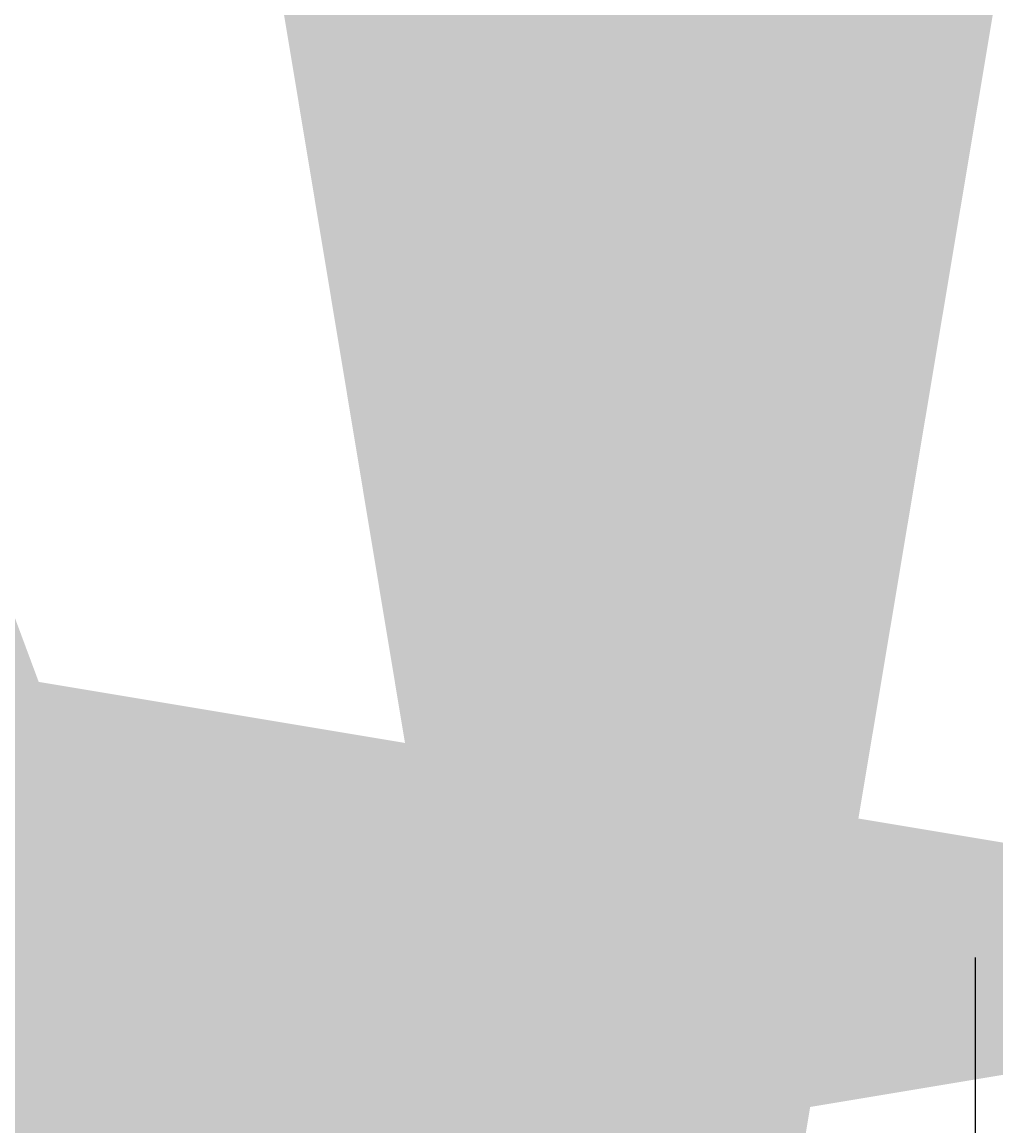
# Model space of a CAD drawing. Units: millimetres. Extents: x -22994 to 29398, y -19990 to 20176.
# Tile 26 of 135: x -44 to 99, y 180 to 341. Entities that reach past the tile are written whole.
import ezdxf

# ---------------------------------------------------------------- set-up
doc = ezdxf.new("R2010")
doc.units = ezdxf.units.MM
doc.header["$MEASUREMENT"] = 0
doc.layers.add('M-DIMS', color=2, linetype='Continuous', lineweight=18)
doc.styles.get("Standard").update_dxf_attribs({"font": 'arial.ttf'})
doc.dimstyles.get("Standard").update_dxf_attribs({"dimtxt": 0.18, "dimasz": 10000, "dimexe": 0.18, "dimexo": 0.0625, "dimgap": 0.09, "dimtad": 0, "dimtih": 1, "dimtoh": 1, "dimdec": 0, "dimzin": 0, "dimdsep": 46, "dimtxsty": 'Standard', "dimcen": 0.09, "dimadec": 0, "dimazin": 0, "dimtfac": 1, "dimtdec": 0, "dimtofl": 0, "dimtmove": 0, "dimatfit": 3, "dimfxl": 1, "dimtolj": 1, "dimtzin": 0, "dimlwd": 30, "dimarcsym": 0})

# ---------------------------------------------------------------- blocks, each defined once
blk = doc.blocks.new('*D2')
at = {"layer": 'Defpoints', "color": 0, "transparency": 16777216}
for p in [(6.68, 10.27), (290.85, 10.27), (290.85, -5.08)]:
    blk.add_point(p, dxfattribs=at)
at = {"layer": 'M-DIMS', "color": 0, "lineweight": -2, "transparency": 16777216}
for p, q in [((6.68, 10.21), (6.68, -5.26)), ((290.85, 10.21), (290.85, -5.26))]:
    blk.add_line(p, q, dxfattribs=at)
at = {"layer": 'M-DIMS', "color": 0, "lineweight": 30, "transparency": 16777216}
for p, q in [((-9993.32, -5.08), (-19993.32, -5.08)), ((10290.85, -5.08), (20290.85, -5.08))]:
    blk.add_line(p, q, dxfattribs=at)
at = {"layer": 'M-DIMS', "color": 0, "transparency": 16777216}
for points in [[(-9993.32, 1661.59), (-9993.32, -1671.75), (6.68, -5.08)], [(10290.85, 1661.59), (10290.85, -1671.75), (290.85, -5.08)]]:
    blk.add_solid(points, dxfattribs=at)
at = {"layer": 'M-DIMS', "color": 0, "transparency": 16777216, "insert": (148.76, -5.08), "char_height": 0.18, "attachment_point": 5}
blk.add_mtext('\\A1;284.2', dxfattribs=at)
blk = doc.blocks.new('*D3')
at = {"layer": 'Defpoints', "color": 0, "transparency": 16777216}
for p in [(110.26, 204.17), (110.26, 176.37), (95.83, 127.97)]:
    blk.add_point(p, dxfattribs=at)
at = {"layer": 'M-DIMS', "color": 0, "lineweight": 30, "transparency": 16777216}
for p, q in [((-9904.17, 204.17), (-19904.17, 204.17)), ((10110.26, 204.17), (20110.26, 204.17))]:
    blk.add_line(p, q, dxfattribs=at)
at = {"layer": 'M-DIMS', "color": 0, "lineweight": -2, "transparency": 16777216}
for p, q in [((95.83, 128.03), (95.83, 204.35)), ((110.26, 176.43), (110.26, 204.35))]:
    blk.add_line(p, q, dxfattribs=at)
at = {"layer": 'M-DIMS', "color": 0, "transparency": 16777216}
for points in [[(-9904.17, 1870.83), (-9904.17, -1462.5), (95.83, 204.17)], [(10110.26, 1870.83), (10110.26, -1462.5), (110.26, 204.17)]]:
    blk.add_solid(points, dxfattribs=at)
at = {"layer": 'M-DIMS', "color": 0, "transparency": 16777216, "insert": (103.05, 204.17), "char_height": 0.18, "attachment_point": 5}
blk.add_mtext('\\A1;14.432', dxfattribs=at)
blk = doc.blocks.new('*D4')
at = {"layer": 'Defpoints', "color": 0, "transparency": 16777216}
for p in [(116.26, 204.17), (110.26, 176.37), (116.26, 176.37)]:
    blk.add_point(p, dxfattribs=at)
at = {"layer": 'M-DIMS', "color": 0, "lineweight": 30, "transparency": 16777216}
for p, q in [((-9889.74, 204.17), (-19889.74, 204.17)), ((10116.26, 204.17), (20116.26, 204.17))]:
    blk.add_line(p, q, dxfattribs=at)
at = {"layer": 'M-DIMS', "color": 0, "lineweight": -2, "transparency": 16777216}
for p, q in [((110.26, 176.43), (110.26, 204.35)), ((116.26, 176.43), (116.26, 204.35))]:
    blk.add_line(p, q, dxfattribs=at)
at = {"layer": 'M-DIMS', "color": 0, "transparency": 16777216}
for points in [[(-9889.74, 1870.83), (-9889.74, -1462.5), (110.26, 204.17)], [(10116.26, 1870.83), (10116.26, -1462.5), (116.26, 204.17)]]:
    blk.add_solid(points, dxfattribs=at)
at = {"layer": 'M-DIMS', "color": 0, "transparency": 16777216, "insert": (113.26, 204.17), "char_height": 0.18, "attachment_point": 5}
blk.add_mtext('\\A1;6', dxfattribs=at)
blk = doc.blocks.new('*D5')
at = {"layer": 'Defpoints', "color": 0, "transparency": 16777216}
for p in [(181.26, 204.17), (116.26, 176.37), (181.26, 176.37)]:
    blk.add_point(p, dxfattribs=at)
at = {"layer": 'M-DIMS', "color": 0, "lineweight": 30, "transparency": 16777216}
for p, q in [((-9883.74, 204.17), (-19883.74, 204.17)), ((10181.26, 204.17), (20181.26, 204.17))]:
    blk.add_line(p, q, dxfattribs=at)
at = {"layer": 'M-DIMS', "color": 0, "lineweight": -2, "transparency": 16777216}
for p, q in [((116.26, 176.43), (116.26, 204.35)), ((181.26, 176.43), (181.26, 204.35))]:
    blk.add_line(p, q, dxfattribs=at)
at = {"layer": 'M-DIMS', "color": 0, "transparency": 16777216}
for points in [[(-9883.74, 1870.83), (-9883.74, -1462.5), (116.26, 204.17)], [(10181.26, 1870.83), (10181.26, -1462.5), (181.26, 204.17)]]:
    blk.add_solid(points, dxfattribs=at)
at = {"layer": 'M-DIMS', "color": 0, "transparency": 16777216, "insert": (148.76, 204.17), "char_height": 0.18, "attachment_point": 5}
blk.add_mtext('\\A1;65', dxfattribs=at)
blk = doc.blocks.new('*D6')
at = {"layer": 'Defpoints', "color": 0, "transparency": 16777216}
for p in [(187.26, 204.17), (181.26, 176.37), (187.26, 176.37)]:
    blk.add_point(p, dxfattribs=at)
at = {"layer": 'M-DIMS', "color": 0, "lineweight": 30, "transparency": 16777216}
for p, q in [((-9818.74, 204.17), (-19818.74, 204.17)), ((10187.26, 204.17), (20187.26, 204.17))]:
    blk.add_line(p, q, dxfattribs=at)
at = {"layer": 'M-DIMS', "color": 0, "lineweight": -2, "transparency": 16777216}
for p, q in [((181.26, 176.43), (181.26, 204.35)), ((187.26, 176.43), (187.26, 204.35))]:
    blk.add_line(p, q, dxfattribs=at)
at = {"layer": 'M-DIMS', "color": 0, "transparency": 16777216}
for points in [[(-9818.74, 1870.83), (-9818.74, -1462.5), (181.26, 204.17)], [(10187.26, 1870.83), (10187.26, -1462.5), (187.26, 204.17)]]:
    blk.add_solid(points, dxfattribs=at)
at = {"layer": 'M-DIMS', "color": 0, "transparency": 16777216, "insert": (184.26, 204.17), "char_height": 0.18, "attachment_point": 5}
blk.add_mtext('\\A1;6', dxfattribs=at)
blk = doc.blocks.new('*D7')
at = {"layer": 'Defpoints', "color": 0, "transparency": 16777216}
for p in [(201.7, 204.17), (187.26, 176.37), (201.7, 127.97)]:
    blk.add_point(p, dxfattribs=at)
at = {"layer": 'M-DIMS', "color": 0, "lineweight": 30, "transparency": 16777216}
for p, q in [((-9812.74, 204.17), (-19812.74, 204.17)), ((10201.7, 204.17), (20201.7, 204.17))]:
    blk.add_line(p, q, dxfattribs=at)
at = {"layer": 'M-DIMS', "color": 0, "lineweight": -2, "transparency": 16777216}
for p, q in [((187.26, 176.43), (187.26, 204.35)), ((201.7, 128.03), (201.7, 204.35))]:
    blk.add_line(p, q, dxfattribs=at)
at = {"layer": 'M-DIMS', "color": 0, "transparency": 16777216}
for points in [[(-9812.74, 1870.83), (-9812.74, -1462.5), (187.26, 204.17)], [(10201.7, 1870.83), (10201.7, -1462.5), (201.7, 204.17)]]:
    blk.add_solid(points, dxfattribs=at)
at = {"layer": 'M-DIMS', "color": 0, "transparency": 16777216, "insert": (194.48, 204.17), "char_height": 0.18, "attachment_point": 5}
blk.add_mtext('\\A1;14.432', dxfattribs=at)
blk = doc.blocks.new('*D8')
at = {"layer": 'Defpoints', "color": 0, "transparency": 16777216}
for p in [(227.65, 204.17), (227.65, 146.73), (201.7, 127.97)]:
    blk.add_point(p, dxfattribs=at)
at = {"layer": 'M-DIMS', "color": 0, "lineweight": 30, "transparency": 16777216}
for p, q in [((-9798.3, 204.17), (-19798.3, 204.17)), ((10227.65, 204.17), (20227.65, 204.17))]:
    blk.add_line(p, q, dxfattribs=at)
at = {"layer": 'M-DIMS', "color": 0, "lineweight": -2, "transparency": 16777216}
for p, q in [((201.7, 128.03), (201.7, 204.35)), ((227.65, 146.79), (227.65, 204.35))]:
    blk.add_line(p, q, dxfattribs=at)
at = {"layer": 'M-DIMS', "color": 0, "transparency": 16777216}
for points in [[(-9798.3, 1870.83), (-9798.3, -1462.5), (201.7, 204.17)], [(10227.65, 1870.83), (10227.65, -1462.5), (227.65, 204.17)]]:
    blk.add_solid(points, dxfattribs=at)
at = {"layer": 'M-DIMS', "color": 0, "transparency": 16777216, "insert": (214.67, 204.17), "char_height": 0.18, "attachment_point": 5}
blk.add_mtext('\\A1;25.95', dxfattribs=at)
blk = doc.blocks.new('*D9')
at = {"layer": 'Defpoints', "color": 0, "transparency": 16777216}
for p in [(187.26, 176.37), (306.2, 176.37), (290.85, 10.27)]:
    blk.add_point(p, dxfattribs=at)
at = {"layer": 'M-DIMS', "color": 0, "lineweight": 30, "transparency": 16777216}
for p, q in [((306.2, 10176.37), (306.2, 20176.37)), ((306.2, -9989.73), (306.2, -19989.73))]:
    blk.add_line(p, q, dxfattribs=at)
at = {"layer": 'M-DIMS', "color": 0, "lineweight": -2, "transparency": 16777216}
for p, q in [((187.33, 176.37), (306.38, 176.37)), ((290.91, 10.27), (306.38, 10.27))]:
    blk.add_line(p, q, dxfattribs=at)
at = {"layer": 'M-DIMS', "color": 0, "transparency": 16777216}
for points in [[(-1360.46, 10176.37), (1972.87, 10176.37), (306.2, 176.37)], [(-1360.46, -9989.73), (1972.87, -9989.73), (306.2, 10.27)]]:
    blk.add_solid(points, dxfattribs=at)
at = {"layer": 'M-DIMS', "color": 0, "transparency": 16777216, "insert": (306.2, 93.32), "char_height": 0.18, "attachment_point": 5}
blk.add_mtext('\\A1;166.1', dxfattribs=at)
blk = doc.blocks.new('*D10')
at = {"layer": 'Defpoints', "color": 0, "transparency": 16777216}
for p in [(125.65, 136.07), (133.35, 136.07), (133.35, -5.08)]:
    blk.add_point(p, dxfattribs=at)
at = {"layer": 'M-DIMS', "color": 0, "lineweight": -2, "transparency": 16777216}
for p, q in [((125.65, 136.01), (125.65, -5.26)), ((133.35, 136.01), (133.35, -5.26))]:
    blk.add_line(p, q, dxfattribs=at)
at = {"layer": 'M-DIMS', "color": 0, "lineweight": 30, "transparency": 16777216}
for p, q in [((-9874.35, -5.08), (-19874.35, -5.08)), ((10133.35, -5.08), (20133.35, -5.08))]:
    blk.add_line(p, q, dxfattribs=at)
at = {"layer": 'M-DIMS', "color": 0, "transparency": 16777216}
for points in [[(-9874.35, 1661.59), (-9874.35, -1671.75), (125.65, -5.08)], [(10133.35, 1661.59), (10133.35, -1671.75), (133.35, -5.08)]]:
    blk.add_solid(points, dxfattribs=at)
at = {"layer": 'M-DIMS', "color": 0, "transparency": 16777216, "insert": (129.5, -5.08), "char_height": 0.18, "attachment_point": 5}
blk.add_mtext('\\A1;7.696', dxfattribs=at)
blk = doc.blocks.new('*D11')
at = {"layer": 'Defpoints', "color": 0, "transparency": 16777216}
for p in [(133.35, 136.07), (135.65, 136.07), (135.65, -5.08)]:
    blk.add_point(p, dxfattribs=at)
at = {"layer": 'M-DIMS', "color": 0, "lineweight": -2, "transparency": 16777216}
for p, q in [((133.35, 136.01), (133.35, -5.26)), ((135.65, 136.01), (135.65, -5.26))]:
    blk.add_line(p, q, dxfattribs=at)
at = {"layer": 'M-DIMS', "color": 0, "lineweight": 30, "transparency": 16777216}
for p, q in [((-9866.65, -5.08), (-19866.65, -5.08)), ((10135.65, -5.08), (20135.65, -5.08))]:
    blk.add_line(p, q, dxfattribs=at)
at = {"layer": 'M-DIMS', "color": 0, "transparency": 16777216}
for points in [[(-9866.65, 1661.59), (-9866.65, -1671.75), (133.35, -5.08)], [(10135.65, 1661.59), (10135.65, -1671.75), (135.65, -5.08)]]:
    blk.add_solid(points, dxfattribs=at)
at = {"layer": 'M-DIMS', "color": 0, "transparency": 16777216, "insert": (134.5, -5.08), "char_height": 0.18, "attachment_point": 5}
blk.add_mtext('\\A1;2.304', dxfattribs=at)
blk = doc.blocks.new('*D12')
at = {"layer": 'Defpoints', "color": 0, "transparency": 16777216}
for p in [(135.65, 136.07), (145.65, 136.07), (145.65, -5.08)]:
    blk.add_point(p, dxfattribs=at)
at = {"layer": 'M-DIMS', "color": 0, "lineweight": -2, "transparency": 16777216}
for p, q in [((135.65, 136.01), (135.65, -5.26)), ((145.65, 136.01), (145.65, -5.26))]:
    blk.add_line(p, q, dxfattribs=at)
at = {"layer": 'M-DIMS', "color": 0, "lineweight": 30, "transparency": 16777216}
for p, q in [((-9864.35, -5.08), (-19864.35, -5.08)), ((10145.65, -5.08), (20145.65, -5.08))]:
    blk.add_line(p, q, dxfattribs=at)
at = {"layer": 'M-DIMS', "color": 0, "transparency": 16777216}
for points in [[(-9864.35, 1661.59), (-9864.35, -1671.75), (135.65, -5.08)], [(10145.65, 1661.59), (10145.65, -1671.75), (145.65, -5.08)]]:
    blk.add_solid(points, dxfattribs=at)
at = {"layer": 'M-DIMS', "color": 0, "transparency": 16777216, "insert": (140.65, -5.08), "char_height": 0.18, "attachment_point": 5}
blk.add_mtext('\\A1;10', dxfattribs=at)
blk = doc.blocks.new('*D13')
at = {"layer": 'Defpoints', "color": 0, "transparency": 16777216}
for p in [(145.65, 136.07), (155.65, 136.07), (155.65, -5.08)]:
    blk.add_point(p, dxfattribs=at)
at = {"layer": 'M-DIMS', "color": 0, "lineweight": -2, "transparency": 16777216}
for p, q in [((145.65, 136.01), (145.65, -5.26)), ((155.65, 136.01), (155.65, -5.26))]:
    blk.add_line(p, q, dxfattribs=at)
at = {"layer": 'M-DIMS', "color": 0, "lineweight": 30, "transparency": 16777216}
for p, q in [((-9854.35, -5.08), (-19854.35, -5.08)), ((10155.65, -5.08), (20155.65, -5.08))]:
    blk.add_line(p, q, dxfattribs=at)
at = {"layer": 'M-DIMS', "color": 0, "transparency": 16777216}
for points in [[(-9854.35, 1661.59), (-9854.35, -1671.75), (145.65, -5.08)], [(10155.65, 1661.59), (10155.65, -1671.75), (155.65, -5.08)]]:
    blk.add_solid(points, dxfattribs=at)
at = {"layer": 'M-DIMS', "color": 0, "transparency": 16777216, "insert": (150.65, -5.08), "char_height": 0.18, "attachment_point": 5}
blk.add_mtext('\\A1;10', dxfattribs=at)
blk = doc.blocks.new('*D14')
at = {"layer": 'Defpoints', "color": 0, "transparency": 16777216}
for p in [(155.65, 136.07), (165.65, 136.07), (165.65, -5.08)]:
    blk.add_point(p, dxfattribs=at)
at = {"layer": 'M-DIMS', "color": 0, "lineweight": -2, "transparency": 16777216}
for p, q in [((155.65, 136.01), (155.65, -5.26)), ((165.65, 136.01), (165.65, -5.26))]:
    blk.add_line(p, q, dxfattribs=at)
at = {"layer": 'M-DIMS', "color": 0, "lineweight": 30, "transparency": 16777216}
for p, q in [((-9844.35, -5.08), (-19844.35, -5.08)), ((10165.65, -5.08), (20165.65, -5.08))]:
    blk.add_line(p, q, dxfattribs=at)
at = {"layer": 'M-DIMS', "color": 0, "transparency": 16777216}
for points in [[(-9844.35, 1661.59), (-9844.35, -1671.75), (155.65, -5.08)], [(10165.65, 1661.59), (10165.65, -1671.75), (165.65, -5.08)]]:
    blk.add_solid(points, dxfattribs=at)
at = {"layer": 'M-DIMS', "color": 0, "transparency": 16777216, "insert": (160.65, -5.08), "char_height": 0.18, "attachment_point": 5}
blk.add_mtext('\\A1;10', dxfattribs=at)
blk = doc.blocks.new('*D15')
at = {"layer": 'Defpoints', "color": 0, "transparency": 16777216}
for p in [(173.35, 154.79), (173.35, 136.07), (306.2, 136.07)]:
    blk.add_point(p, dxfattribs=at)
at = {"layer": 'M-DIMS', "color": 0, "lineweight": 30, "transparency": 16777216}
for p, q in [((306.2, 10154.79), (306.2, 20154.79)), ((306.2, -9863.93), (306.2, -19863.93))]:
    blk.add_line(p, q, dxfattribs=at)
at = {"layer": 'M-DIMS', "color": 0, "lineweight": -2, "transparency": 16777216}
for p, q in [((173.41, 154.79), (306.38, 154.79)), ((173.41, 136.07), (306.38, 136.07))]:
    blk.add_line(p, q, dxfattribs=at)
at = {"layer": 'M-DIMS', "color": 0, "transparency": 16777216}
for points in [[(-1360.46, 10154.79), (1972.87, 10154.79), (306.2, 154.79)], [(-1360.46, -9863.93), (1972.87, -9863.93), (306.2, 136.07)]]:
    blk.add_solid(points, dxfattribs=at)
at = {"layer": 'M-DIMS', "color": 0, "transparency": 16777216, "insert": (306.2, 145.43), "char_height": 0.18, "attachment_point": 5}
blk.add_mtext('\\A1;18.717', dxfattribs=at)
blk = doc.blocks.new('*D16')
at = {"layer": 'Defpoints', "color": 0, "transparency": 16777216}
for p in [(120.17, 204.17), (110.47, 48.03), (120.17, 48.03)]:
    blk.add_point(p, dxfattribs=at)
at = {"layer": 'M-DIMS', "color": 0, "lineweight": 30, "transparency": 16777216}
for p, q in [((-9889.53, 204.17), (-19889.53, 204.17)), ((10120.17, 204.17), (20120.17, 204.17))]:
    blk.add_line(p, q, dxfattribs=at)
at = {"layer": 'M-DIMS', "color": 0, "lineweight": -2, "transparency": 16777216}
for p, q in [((110.47, 48.1), (110.47, 204.35)), ((120.17, 48.1), (120.17, 204.35))]:
    blk.add_line(p, q, dxfattribs=at)
at = {"layer": 'M-DIMS', "color": 0, "transparency": 16777216}
for points in [[(-9889.53, 1870.83), (-9889.53, -1462.5), (110.47, 204.17)], [(10120.17, 1870.83), (10120.17, -1462.5), (120.17, 204.17)]]:
    blk.add_solid(points, dxfattribs=at)
at = {"layer": 'M-DIMS', "color": 0, "transparency": 16777216, "insert": (115.32, 204.17), "char_height": 0.18, "attachment_point": 5}
blk.add_mtext('\\A1;9.704', dxfattribs=at)
blk = doc.blocks.new('*D17')
at = {"layer": 'Defpoints', "color": 0, "transparency": 16777216}
for p in [(126.17, 204.17), (120.17, 48.03), (126.17, 48.03)]:
    blk.add_point(p, dxfattribs=at)
at = {"layer": 'M-DIMS', "color": 0, "lineweight": 30, "transparency": 16777216}
for p, q in [((-9879.83, 204.17), (-19879.83, 204.17)), ((10126.17, 204.17), (20126.17, 204.17))]:
    blk.add_line(p, q, dxfattribs=at)
at = {"layer": 'M-DIMS', "color": 0, "lineweight": -2, "transparency": 16777216}
for p, q in [((120.17, 48.1), (120.17, 204.35)), ((126.17, 48.1), (126.17, 204.35))]:
    blk.add_line(p, q, dxfattribs=at)
at = {"layer": 'M-DIMS', "color": 0, "transparency": 16777216}
for points in [[(-9879.83, 1870.83), (-9879.83, -1462.5), (120.17, 204.17)], [(10126.17, 1870.83), (10126.17, -1462.5), (126.17, 204.17)]]:
    blk.add_solid(points, dxfattribs=at)
at = {"layer": 'M-DIMS', "color": 0, "transparency": 16777216, "insert": (123.17, 204.17), "char_height": 0.18, "attachment_point": 5}
blk.add_mtext('\\A1;6', dxfattribs=at)
blk = doc.blocks.new('*D18')
at = {"layer": 'Defpoints', "color": 0, "transparency": 16777216}
for p in [(132.17, 204.17), (126.17, 48.03), (132.17, 48.03)]:
    blk.add_point(p, dxfattribs=at)
at = {"layer": 'M-DIMS', "color": 0, "lineweight": 30, "transparency": 16777216}
for p, q in [((-9873.83, 204.17), (-19873.83, 204.17)), ((10132.17, 204.17), (20132.17, 204.17))]:
    blk.add_line(p, q, dxfattribs=at)
at = {"layer": 'M-DIMS', "color": 0, "lineweight": -2, "transparency": 16777216}
for p, q in [((126.17, 48.1), (126.17, 204.35)), ((132.17, 48.1), (132.17, 204.35))]:
    blk.add_line(p, q, dxfattribs=at)
at = {"layer": 'M-DIMS', "color": 0, "transparency": 16777216}
for points in [[(-9873.83, 1870.83), (-9873.83, -1462.5), (126.17, 204.17)], [(10132.17, 1870.83), (10132.17, -1462.5), (132.17, 204.17)]]:
    blk.add_solid(points, dxfattribs=at)
at = {"layer": 'M-DIMS', "color": 0, "transparency": 16777216, "insert": (129.17, 204.17), "char_height": 0.18, "attachment_point": 5}
blk.add_mtext('\\A1;6', dxfattribs=at)
blk = doc.blocks.new('*D19')
at = {"layer": 'Defpoints', "color": 0, "transparency": 16777216}
for p in [(138.17, 204.17), (132.17, 48.03), (138.17, 48.03)]:
    blk.add_point(p, dxfattribs=at)
at = {"layer": 'M-DIMS', "color": 0, "lineweight": 30, "transparency": 16777216}
for p, q in [((-9867.83, 204.17), (-19867.83, 204.17)), ((10138.17, 204.17), (20138.17, 204.17))]:
    blk.add_line(p, q, dxfattribs=at)
at = {"layer": 'M-DIMS', "color": 0, "lineweight": -2, "transparency": 16777216}
for p, q in [((132.17, 48.1), (132.17, 204.35)), ((138.17, 48.1), (138.17, 204.35))]:
    blk.add_line(p, q, dxfattribs=at)
at = {"layer": 'M-DIMS', "color": 0, "transparency": 16777216}
for points in [[(-9867.83, 1870.83), (-9867.83, -1462.5), (132.17, 204.17)], [(10138.17, 1870.83), (10138.17, -1462.5), (138.17, 204.17)]]:
    blk.add_solid(points, dxfattribs=at)
at = {"layer": 'M-DIMS', "color": 0, "transparency": 16777216, "insert": (135.17, 204.17), "char_height": 0.18, "attachment_point": 5}
blk.add_mtext('\\A1;6', dxfattribs=at)
blk = doc.blocks.new('*D20')
at = {"layer": 'Defpoints', "color": 0, "transparency": 16777216}
for p in [(144.17, 204.17), (138.17, 48.03), (144.17, 48.03)]:
    blk.add_point(p, dxfattribs=at)
at = {"layer": 'M-DIMS', "color": 0, "lineweight": 30, "transparency": 16777216}
for p, q in [((-9861.83, 204.17), (-19861.83, 204.17)), ((10144.17, 204.17), (20144.17, 204.17))]:
    blk.add_line(p, q, dxfattribs=at)
at = {"layer": 'M-DIMS', "color": 0, "lineweight": -2, "transparency": 16777216}
for p, q in [((138.17, 48.1), (138.17, 204.35)), ((144.17, 48.1), (144.17, 204.35))]:
    blk.add_line(p, q, dxfattribs=at)
at = {"layer": 'M-DIMS', "color": 0, "transparency": 16777216}
for points in [[(-9861.83, 1870.83), (-9861.83, -1462.5), (138.17, 204.17)], [(10144.17, 1870.83), (10144.17, -1462.5), (144.17, 204.17)]]:
    blk.add_solid(points, dxfattribs=at)
at = {"layer": 'M-DIMS', "color": 0, "transparency": 16777216, "insert": (141.17, 204.17), "char_height": 0.18, "attachment_point": 5}
blk.add_mtext('\\A1;6', dxfattribs=at)
blk = doc.blocks.new('*D21')
at = {"layer": 'Defpoints', "color": 0, "transparency": 16777216}
for p in [(149.12, 204.17), (144.17, 48.03), (149.12, 48.03)]:
    blk.add_point(p, dxfattribs=at)
at = {"layer": 'M-DIMS', "color": 0, "lineweight": 30, "transparency": 16777216}
for p, q in [((-9855.83, 204.17), (-19855.83, 204.17)), ((10149.12, 204.17), (20149.12, 204.17))]:
    blk.add_line(p, q, dxfattribs=at)
at = {"layer": 'M-DIMS', "color": 0, "lineweight": -2, "transparency": 16777216}
for p, q in [((144.17, 48.1), (144.17, 204.35)), ((149.12, 48.1), (149.12, 204.35))]:
    blk.add_line(p, q, dxfattribs=at)
at = {"layer": 'M-DIMS', "color": 0, "transparency": 16777216}
for points in [[(-9855.83, 1870.83), (-9855.83, -1462.5), (144.17, 204.17)], [(10149.12, 1870.83), (10149.12, -1462.5), (149.12, 204.17)]]:
    blk.add_solid(points, dxfattribs=at)
at = {"layer": 'M-DIMS', "color": 0, "transparency": 16777216, "insert": (146.64, 204.17), "char_height": 0.18, "attachment_point": 5}
blk.add_mtext('\\A1;4.945', dxfattribs=at)
blk = doc.blocks.new('*D22')
at = {"layer": 'Defpoints', "color": 0, "transparency": 16777216}
for p in [(149.12, 30.99), (155.12, 30.99), (155.12, -5.08)]:
    blk.add_point(p, dxfattribs=at)
at = {"layer": 'M-DIMS', "color": 0, "lineweight": -2, "transparency": 16777216}
for p, q in [((149.12, 30.93), (149.12, -5.26)), ((155.12, 30.93), (155.12, -5.26))]:
    blk.add_line(p, q, dxfattribs=at)
at = {"layer": 'M-DIMS', "color": 0, "lineweight": 30, "transparency": 16777216}
for p, q in [((-9850.88, -5.08), (-19850.88, -5.08)), ((10155.12, -5.08), (20155.12, -5.08))]:
    blk.add_line(p, q, dxfattribs=at)
at = {"layer": 'M-DIMS', "color": 0, "transparency": 16777216}
for points in [[(-9850.88, 1661.59), (-9850.88, -1671.75), (149.12, -5.08)], [(10155.12, 1661.59), (10155.12, -1671.75), (155.12, -5.08)]]:
    blk.add_solid(points, dxfattribs=at)
at = {"layer": 'M-DIMS', "color": 0, "transparency": 16777216, "insert": (152.12, -5.08), "char_height": 0.18, "attachment_point": 5}
blk.add_mtext('\\A1;6', dxfattribs=at)
blk = doc.blocks.new('*D23')
at = {"layer": 'Defpoints', "color": 0, "transparency": 16777216}
for p in [(155.12, 30.99), (161.12, 30.99), (161.12, -5.08)]:
    blk.add_point(p, dxfattribs=at)
at = {"layer": 'M-DIMS', "color": 0, "lineweight": -2, "transparency": 16777216}
for p, q in [((155.12, 30.93), (155.12, -5.26)), ((161.12, 30.93), (161.12, -5.26))]:
    blk.add_line(p, q, dxfattribs=at)
at = {"layer": 'M-DIMS', "color": 0, "lineweight": 30, "transparency": 16777216}
for p, q in [((-9844.88, -5.08), (-19844.88, -5.08)), ((10161.12, -5.08), (20161.12, -5.08))]:
    blk.add_line(p, q, dxfattribs=at)
at = {"layer": 'M-DIMS', "color": 0, "transparency": 16777216}
for points in [[(-9844.88, 1661.59), (-9844.88, -1671.75), (155.12, -5.08)], [(10161.12, 1661.59), (10161.12, -1671.75), (161.12, -5.08)]]:
    blk.add_solid(points, dxfattribs=at)
at = {"layer": 'M-DIMS', "color": 0, "transparency": 16777216, "insert": (158.12, -5.08), "char_height": 0.18, "attachment_point": 5}
blk.add_mtext('\\A1;6', dxfattribs=at)
blk = doc.blocks.new('*D24')
at = {"layer": 'Defpoints', "color": 0, "transparency": 16777216}
for p in [(161.12, 30.99), (166.44, 30.99), (166.44, -5.08)]:
    blk.add_point(p, dxfattribs=at)
at = {"layer": 'M-DIMS', "color": 0, "lineweight": -2, "transparency": 16777216}
for p, q in [((161.12, 30.93), (161.12, -5.26)), ((166.44, 30.93), (166.44, -5.26))]:
    blk.add_line(p, q, dxfattribs=at)
at = {"layer": 'M-DIMS', "color": 0, "lineweight": 30, "transparency": 16777216}
for p, q in [((-9838.88, -5.08), (-19838.88, -5.08)), ((10166.44, -5.08), (20166.44, -5.08))]:
    blk.add_line(p, q, dxfattribs=at)
at = {"layer": 'M-DIMS', "color": 0, "transparency": 16777216}
for points in [[(-9838.88, 1661.59), (-9838.88, -1671.75), (161.12, -5.08)], [(10166.44, 1661.59), (10166.44, -1671.75), (166.44, -5.08)]]:
    blk.add_solid(points, dxfattribs=at)
at = {"layer": 'M-DIMS', "color": 0, "transparency": 16777216, "insert": (163.78, -5.08), "char_height": 0.18, "attachment_point": 5}
blk.add_mtext('\\A1;5.323', dxfattribs=at)
blk = doc.blocks.new('*D25')
at = {"layer": 'Defpoints', "color": 0, "transparency": 16777216}
for p in [(166.44, 30.99), (172.44, 30.99), (172.44, -5.08)]:
    blk.add_point(p, dxfattribs=at)
at = {"layer": 'M-DIMS', "color": 0, "lineweight": -2, "transparency": 16777216}
for p, q in [((166.44, 30.93), (166.44, -5.26)), ((172.44, 30.93), (172.44, -5.26))]:
    blk.add_line(p, q, dxfattribs=at)
at = {"layer": 'M-DIMS', "color": 0, "lineweight": 30, "transparency": 16777216}
for p, q in [((-9833.56, -5.08), (-19833.56, -5.08)), ((10172.44, -5.08), (20172.44, -5.08))]:
    blk.add_line(p, q, dxfattribs=at)
at = {"layer": 'M-DIMS', "color": 0, "transparency": 16777216}
for points in [[(-9833.56, 1661.59), (-9833.56, -1671.75), (166.44, -5.08)], [(10172.44, 1661.59), (10172.44, -1671.75), (172.44, -5.08)]]:
    blk.add_solid(points, dxfattribs=at)
at = {"layer": 'M-DIMS', "color": 0, "transparency": 16777216, "insert": (169.44, -5.08), "char_height": 0.18, "attachment_point": 5}
blk.add_mtext('\\A1;6', dxfattribs=at)
blk = doc.blocks.new('*D26')
at = {"layer": 'Defpoints', "color": 0, "transparency": 16777216}
for p in [(172.44, 30.99), (178.44, 30.99), (178.44, -5.08)]:
    blk.add_point(p, dxfattribs=at)
at = {"layer": 'M-DIMS', "color": 0, "lineweight": -2, "transparency": 16777216}
for p, q in [((172.44, 30.93), (172.44, -5.26)), ((178.44, 30.93), (178.44, -5.26))]:
    blk.add_line(p, q, dxfattribs=at)
at = {"layer": 'M-DIMS', "color": 0, "lineweight": 30, "transparency": 16777216}
for p, q in [((-9827.56, -5.08), (-19827.56, -5.08)), ((10178.44, -5.08), (20178.44, -5.08))]:
    blk.add_line(p, q, dxfattribs=at)
at = {"layer": 'M-DIMS', "color": 0, "transparency": 16777216}
for points in [[(-9827.56, 1661.59), (-9827.56, -1671.75), (172.44, -5.08)], [(10178.44, 1661.59), (10178.44, -1671.75), (178.44, -5.08)]]:
    blk.add_solid(points, dxfattribs=at)
at = {"layer": 'M-DIMS', "color": 0, "transparency": 16777216, "insert": (175.44, -5.08), "char_height": 0.18, "attachment_point": 5}
blk.add_mtext('\\A1;6', dxfattribs=at)
blk = doc.blocks.new('*D27')
at = {"layer": 'Defpoints', "color": 0, "transparency": 16777216}
for p in [(178.44, 30.99), (188.12, 30.99), (188.12, -5.08)]:
    blk.add_point(p, dxfattribs=at)
at = {"layer": 'M-DIMS', "color": 0, "lineweight": -2, "transparency": 16777216}
for p, q in [((178.44, 30.93), (178.44, -5.26)), ((188.12, 30.93), (188.12, -5.26))]:
    blk.add_line(p, q, dxfattribs=at)
at = {"layer": 'M-DIMS', "color": 0, "lineweight": 30, "transparency": 16777216}
for p, q in [((-9821.56, -5.08), (-19821.56, -5.08)), ((10188.12, -5.08), (20188.12, -5.08))]:
    blk.add_line(p, q, dxfattribs=at)
at = {"layer": 'M-DIMS', "color": 0, "transparency": 16777216}
for points in [[(-9821.56, 1661.59), (-9821.56, -1671.75), (178.44, -5.08)], [(10188.12, 1661.59), (10188.12, -1671.75), (188.12, -5.08)]]:
    blk.add_solid(points, dxfattribs=at)
at = {"layer": 'M-DIMS', "color": 0, "transparency": 16777216, "insert": (183.28, -5.08), "char_height": 0.18, "attachment_point": 5}
blk.add_mtext('\\A1;9.679', dxfattribs=at)
blk = doc.blocks.new('*D28')
at = {"layer": 'Defpoints', "color": 0, "transparency": 16777216}
for p in [(188.12, 48.03), (306.2, 48.03), (188.12, 30.99)]:
    blk.add_point(p, dxfattribs=at)
at = {"layer": 'M-DIMS', "color": 0, "lineweight": 30, "transparency": 16777216}
for p, q in [((306.2, 10048.03), (306.2, 20048.03)), ((306.2, -9969.01), (306.2, -19969.01))]:
    blk.add_line(p, q, dxfattribs=at)
at = {"layer": 'M-DIMS', "color": 0, "lineweight": -2, "transparency": 16777216}
for p, q in [((188.18, 48.03), (306.38, 48.03)), ((188.18, 30.99), (306.38, 30.99))]:
    blk.add_line(p, q, dxfattribs=at)
at = {"layer": 'M-DIMS', "color": 0, "transparency": 16777216}
for points in [[(-1360.46, 10048.03), (1972.87, 10048.03), (306.2, 48.03)], [(-1360.46, -9969.01), (1972.87, -9969.01), (306.2, 30.99)]]:
    blk.add_solid(points, dxfattribs=at)
at = {"layer": 'M-DIMS', "color": 0, "transparency": 16777216, "insert": (306.2, 39.51), "char_height": 0.18, "attachment_point": 5}
blk.add_mtext('\\A1;17.045', dxfattribs=at)
blk = doc.blocks.new('*D29')
at = {"layer": 'Defpoints', "color": 0, "transparency": 16777216}
for p in [(36.8, 80.04), (64.03, 80.04)]:
    blk.add_point(p, dxfattribs=at)
at = {"layer": 'M-DIMS', "color": 0, "lineweight": -2, "transparency": 16777216}
for p, q in [((50.33, 80.04), (50.51, 80.04)), ((50.42, 79.96), (50.42, 80.14))]:
    blk.add_line(p, q, dxfattribs=at)
at = {"layer": 'M-DIMS', "color": 0, "lineweight": 30, "transparency": 16777216}
blk.add_line((20064.03, 80.03), (10064.03, 80.04), dxfattribs=at)
at = {"layer": 'M-DIMS', "color": 0, "transparency": 16777216}
blk.add_solid([(10064.03, 1746.7), (10064.03, -1586.63), (64.03, 80.04)], dxfattribs=at)
at = {"layer": 'M-DIMS', "color": 0, "transparency": 16777216, "insert": (20064.52, 80.03), "char_height": 0.18, "attachment_point": 5}
blk.add_mtext('\\A1;∅27.23', dxfattribs=at)
blk = doc.blocks.new('*D35')
at = {"layer": 'Defpoints', "color": 0, "transparency": 16777216}
for p in [(21.09, 77.39), (21.84, 76.09)]:
    blk.add_point(p, dxfattribs=at)
at = {"layer": 'M-DIMS', "color": 0, "lineweight": 30, "transparency": 16777216}
for p, q in [((-19938.01, 17421.45), (-9938.01, 17421.45)), ((-9938.01, 17421.45), (-4958.46, 8749.42))]:
    blk.add_line(p, q, dxfattribs=at)
at = {"layer": 'M-DIMS', "color": 0, "lineweight": -2, "transparency": 16777216}
for p, q in [((21.75, 76.09), (21.93, 76.09)), ((21.84, 76), (21.84, 76.18))]:
    blk.add_line(p, q, dxfattribs=at)
at = {"layer": 'M-DIMS', "color": 0, "transparency": 16777216}
blk.add_solid([(-3513.12, 9579.35), (-6403.8, 7919.49), (21.09, 77.39)], dxfattribs=at)
at = {"layer": 'M-DIMS', "color": 0, "transparency": 16777216, "insert": (-19938.35, 17421.45), "char_height": 0.18, "attachment_point": 5}
blk.add_mtext('\\A1;R1.5', dxfattribs=at)
blk = doc.blocks.new('*D36')
at = {"layer": 'Defpoints', "color": 0, "transparency": 16777216}
for p in [(46.39, 31.3), (46.39, 26.59)]:
    blk.add_point(p, dxfattribs=at)
at = {"layer": 'M-DIMS', "color": 0, "lineweight": 30, "transparency": 16777216}
for p, q in [((57.15, 20031.3), (51.77, 10031.3)), ((10057.15, 20031.3), (57.15, 20031.3))]:
    blk.add_line(p, q, dxfattribs=at)
at = {"layer": 'M-DIMS', "color": 0, "lineweight": -2, "transparency": 16777216}
for p, q in [((46.3, 28.95), (46.48, 28.95)), ((46.39, 28.86), (46.39, 29.04))]:
    blk.add_line(p, q, dxfattribs=at)
at = {"layer": 'M-DIMS', "color": 0, "transparency": 16777216}
blk.add_solid([(-1614.9, 10032.2), (1718.44, 10030.41), (46.39, 31.3)], dxfattribs=at)
at = {"layer": 'M-DIMS', "color": 0, "transparency": 16777216, "insert": (10057.55, 20031.3), "char_height": 0.18, "attachment_point": 5}
blk.add_mtext('\\A1;∅4.71', dxfattribs=at)
blk = doc.blocks.new('*D37')
at = {"layer": 'Defpoints', "color": 0, "transparency": 16777216}
for p in [(54.83, 118.61), (59.49, 118.61)]:
    blk.add_point(p, dxfattribs=at)
at = {"layer": 'M-DIMS', "color": 0, "lineweight": -2, "transparency": 16777216}
for p, q in [((57.07, 118.61), (57.25, 118.61)), ((57.16, 118.52), (57.16, 118.7))]:
    blk.add_line(p, q, dxfattribs=at)
at = {"layer": 'M-DIMS', "color": 0, "lineweight": 30, "transparency": 16777216}
blk.add_line((20059.49, 116.25), (10059.49, 117.43), dxfattribs=at)
at = {"layer": 'M-DIMS', "color": 0, "transparency": 16777216}
blk.add_solid([(10059.69, 1784.1), (10059.3, -1549.23), (59.49, 118.61)], dxfattribs=at)
at = {"layer": 'M-DIMS', "color": 0, "transparency": 16777216, "insert": (20059.99, 116.25), "char_height": 0.18, "attachment_point": 5}
blk.add_mtext('\\A1;∅4.659', dxfattribs=at)

msp = doc.modelspace()

# ---------------------------------------------------------------- dimensions: what is measured, and where the dimension line sits
at = {"layer": 'M-DIMS'}
for base, p1, p2, override, picture, middle in [((306.202, 176.3662), (290.852, 10.2713), (187.2647, 176.3662), {"dimdec": 1, "dimlfac": 1, "dimrnd": 0, "dimzin": 0, "dimdsep": 46, "dimlunit": 2}, '*D9', (306.202, 93.3187)), ((306.202, 136.0713), (173.3459, 154.788), (173.3459, 136.0713), {"dimdec": 3, "dimlfac": 1, "dimrnd": 0, "dimzin": 0, "dimdsep": 46, "dimlunit": 2}, '*D15', (306.202, 145.4297)), ((306.202, 48.0349), (188.1175, 30.9895), (188.1175, 48.0349), {"dimdec": 3, "dimlfac": 1, "dimrnd": 0, "dimzin": 0, "dimdsep": 46, "dimlunit": 2}, '*D28', (306.202, 39.5122))]:
    dim = msp.add_linear_dim(base=base, p1=p1, p2=p2, angle=90, dimstyle='Standard', override=override, dxfattribs=at)
    dim.commit()
    dim.dimension.update_dxf_attribs({"geometry": picture, "text_midpoint": middle})
dim = msp.add_diameter_dim_2p(p1=(46.3875, 26.5934), p2=(46.39, 31.3035), dimstyle='Standard', override={"dimdec": 2, "dimlfac": 1, "dimrnd": 0, "dimzin": 0, "dimdsep": 46, "dimlunit": 2}, dxfattribs=at)
dim.commit()
dim.dimension.update_dxf_attribs({"geometry": '*D36', "text_midpoint": (10057.5542, 20031.3006), "dimtype": 163})
dim = msp.add_radius_dim(center=(21.8402, 76.0922), mpoint=(21.0933, 77.393), dimstyle='Standard', override={"dimdec": 1, "dimlfac": 1, "dimrnd": 0, "dimzin": 0, "dimdsep": 46, "dimlunit": 2}, dxfattribs=at)
dim.commit()
dim.dimension.update_dxf_attribs({"geometry": '*D35', "text_midpoint": (-19938.3541, 17421.4466)})
for base, p1, p2, override, picture, middle in [((110.2647, 204.1654), (95.8327, 127.967), (110.2647, 176.3662), {"dimdec": 3, "dimlfac": 1, "dimrnd": 0, "dimzin": 0, "dimdsep": 46, "dimlunit": 2}, '*D3', (103.0487, 204.1654)), ((116.2647, 204.1654), (110.2647, 176.3662), (116.2647, 176.3662), {"dimdec": 0, "dimlfac": 1, "dimrnd": 0, "dimzin": 0, "dimdsep": 46, "dimlunit": 2}, '*D4', (113.2647, 204.1654)), ((120.1702, 204.1654), (110.4658, 48.0349), (120.1702, 48.0349), {"dimdec": 3, "dimlfac": 1, "dimrnd": 0, "dimzin": 0, "dimdsep": 46, "dimlunit": 2}, '*D16', (115.318, 204.1654)), ((181.2647, 204.1654), (116.2647, 176.3662), (181.2647, 176.3662), {"dimdec": 0, "dimlfac": 1, "dimrnd": 0, "dimzin": 0, "dimdsep": 46, "dimlunit": 2}, '*D5', (148.7647, 204.1654)), ((126.1702, 204.1654), (120.1702, 48.0349), (126.1702, 48.0349), {"dimdec": 0, "dimlfac": 1, "dimrnd": 0, "dimzin": 0, "dimdsep": 46, "dimlunit": 2}, '*D17', (123.1702, 204.1654)), ((132.1702, 204.1654), (126.1702, 48.0349), (132.1702, 48.0349), {"dimdec": 0, "dimlfac": 1, "dimrnd": 0, "dimzin": 0, "dimdsep": 46, "dimlunit": 2}, '*D18', (129.1702, 204.1654)), ((138.1702, 204.1654), (132.1702, 48.0349), (138.1702, 48.0349), {"dimdec": 0, "dimlfac": 1, "dimrnd": 0, "dimzin": 0, "dimdsep": 46, "dimlunit": 2}, '*D19', (135.1702, 204.1654)), ((144.1702, 204.1654), (138.1702, 48.0349), (144.1702, 48.0349), {"dimdec": 0, "dimlfac": 1, "dimrnd": 0, "dimzin": 0, "dimdsep": 46, "dimlunit": 2}, '*D20', (141.1702, 204.1654)), ((149.11567, 204.16539), (144.17023, 48.03494), (149.11567, 48.03494), {"dimdec": 3, "dimlfac": 1, "dimrnd": 0, "dimzin": 0, "dimdsep": 46, "dimlunit": 2}, '*D21', (146.64295, 204.16539)), ((187.2647, 204.1654), (181.2647, 176.3662), (187.2647, 176.3662), {"dimdec": 0, "dimlfac": 1, "dimrnd": 0, "dimzin": 0, "dimdsep": 46, "dimlunit": 2}, '*D6', (184.2647, 204.1654)), ((201.6967, 204.1654), (187.2647, 176.3662), (201.6967, 127.967), {"dimdec": 3, "dimlfac": 1, "dimrnd": 0, "dimzin": 0, "dimdsep": 46, "dimlunit": 2}, '*D7', (194.4807, 204.1654)), ((227.6485, 204.1654), (201.6967, 127.967), (227.6485, 146.7296), {"dimdec": 2, "dimlfac": 1, "dimrnd": 0, "dimzin": 0, "dimdsep": 46, "dimlunit": 2}, '*D8', (214.6726, 204.1654)), ((290.852, -5.0787), (6.6773, 10.2713), (290.852, 10.2713), {"dimdec": 1, "dimlfac": 1, "dimrnd": 0, "dimzin": 0, "dimdsep": 46, "dimlunit": 2}, '*D2', (148.7647, -5.0787)), ((133.3459, -5.0787), (125.6498, 136.0713), (133.3459, 136.0713), {"dimdec": 3, "dimlfac": 1, "dimrnd": 0, "dimzin": 0, "dimdsep": 46, "dimlunit": 2}, '*D10', (129.4978, -5.0787)), ((135.6498, -5.0787), (133.3459, 136.0713), (135.6498, 136.0713), {"dimdec": 3, "dimlfac": 1, "dimrnd": 0, "dimzin": 0, "dimdsep": 46, "dimlunit": 2}, '*D11', (134.4978, -5.0787)), ((145.6498, -5.0787), (135.6498, 136.0713), (145.6498, 136.0713), {"dimdec": 0, "dimlfac": 1, "dimrnd": 0, "dimzin": 0, "dimdsep": 46, "dimlunit": 2}, '*D12', (140.6498, -5.0787)), ((155.6498, -5.0787), (145.6498, 136.0713), (155.6498, 136.0713), {"dimdec": 0, "dimlfac": 1, "dimrnd": 0, "dimzin": 0, "dimdsep": 46, "dimlunit": 2}, '*D13', (150.6498, -5.0787)), ((155.1157, -5.0787), (149.1157, 30.9895), (155.1157, 30.9895), {"dimdec": 0, "dimlfac": 1, "dimrnd": 0, "dimzin": 0, "dimdsep": 46, "dimlunit": 2}, '*D22', (152.1157, -5.0787)), ((161.1157, -5.0787), (155.1157, 30.9895), (161.1157, 30.9895), {"dimdec": 0, "dimlfac": 1, "dimrnd": 0, "dimzin": 0, "dimdsep": 46, "dimlunit": 2}, '*D23', (158.1157, -5.0787)), ((165.6498, -5.0787), (155.6498, 136.0713), (165.6498, 136.0713), {"dimdec": 0, "dimlfac": 1, "dimrnd": 0, "dimzin": 0, "dimdsep": 46, "dimlunit": 2}, '*D14', (160.6498, -5.0787)), ((166.4387, -5.0787), (161.1157, 30.9895), (166.4387, 30.9895), {"dimdec": 3, "dimlfac": 1, "dimrnd": 0, "dimzin": 0, "dimdsep": 46, "dimlunit": 2}, '*D24', (163.7772, -5.0787)), ((172.4387, -5.0787), (166.4387, 30.9895), (172.4387, 30.9895), {"dimdec": 0, "dimlfac": 1, "dimrnd": 0, "dimzin": 0, "dimdsep": 46, "dimlunit": 2}, '*D25', (169.4387, -5.0787)), ((178.4387, -5.0787), (172.4387, 30.9895), (178.4387, 30.9895), {"dimdec": 0, "dimlfac": 1, "dimrnd": 0, "dimzin": 0, "dimdsep": 46, "dimlunit": 2}, '*D26', (175.4387, -5.0787)), ((188.1175, -5.0787), (178.4387, 30.9895), (188.1175, 30.9895), {"dimdec": 3, "dimlfac": 1, "dimrnd": 0, "dimzin": 0, "dimdsep": 46, "dimlunit": 2}, '*D27', (183.2781, -5.0787))]:
    dim = msp.add_linear_dim(base=base, p1=p1, p2=p2, dimstyle='Standard', override=override, dxfattribs=at)
    dim.commit()
    dim.dimension.update_dxf_attribs({"geometry": picture, "text_midpoint": middle})
for p1, p2, override, picture, middle in [((54.8343, 118.6145), (59.4936, 118.614), {"dimdec": 3, "dimlfac": 1, "dimrnd": 0, "dimzin": 0, "dimdsep": 46, "dimlunit": 2}, '*D37', (20059.4934, 116.2531)), ((36.8006, 80.045), (64.0296, 80.045), {"dimdec": 2, "dimlfac": 1, "dimrnd": 0, "dimzin": 0, "dimdsep": 46, "dimlunit": 2}, '*D29', (20064.0296, 80.0303))]:
    dim = msp.add_diameter_dim_2p(p1=p1, p2=p2, dimstyle='Standard', override=override, dxfattribs=at)
    dim.commit()
    dim.dimension.update_dxf_attribs({"geometry": picture, "text_midpoint": middle})

doc.saveas('drawing.dxf')
